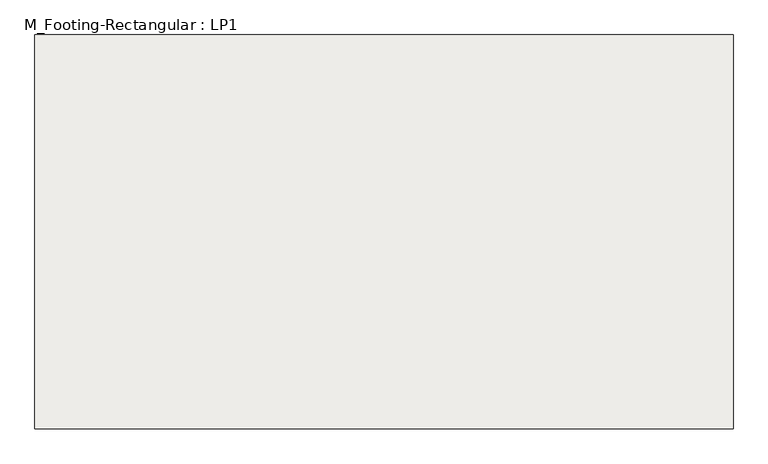
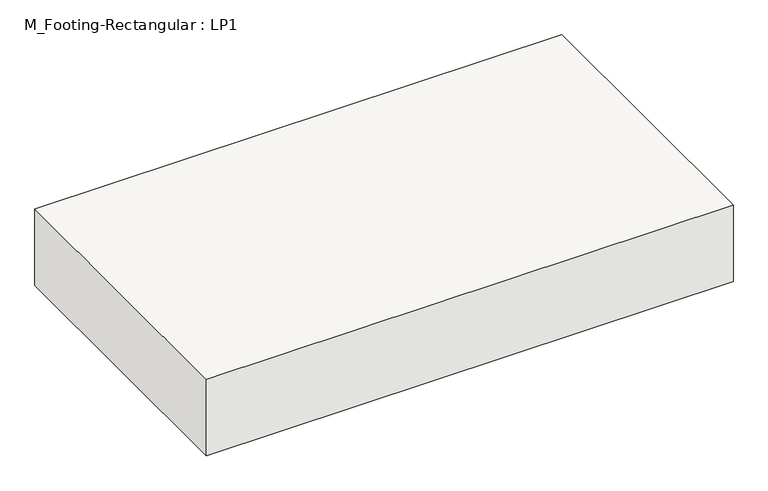
"""IFC4 building model written with IfcOpenShell, lengths in millimetres: slab geometry, M_Footing-Rectangular : LP1."""

from ifc_helpers import new_model, si_unit, frame, origin, place, context, project, spatial, polyline, outline, extrude, source, transform, mapped, element, save


def m_footing_rectangular_lp1_02c7f121(model_context):
    return source(origin(), model_context, "Body", "SweptSolid", [
        extrude(outline(polyline([(1485.9, 838.2), (1485.9, -838.2), (-1485.9, -838.2), (-1485.9, 838.2), (1485.9, 838.2)])), frame((0.0, 0.0, -457.2), z_axis=(0.0, 0.0, 1.0), x_axis=(1.0, 0.0, 0.0)), (0.0, 0.0, 1.0), 457.2),
    ])


if __name__ == "__main__":
    model = new_model("IFC4")
    model_context = context("Model", 3, world=origin())
    ifc_project = project(units=[si_unit("LENGTHUNIT", "METRE", prefix="MILLI")], contexts=[model_context])
    site = spatial("IfcSite", under=ifc_project)
    building = spatial("IfcBuilding", under=site)
    placement = place(None, origin())
    m_footing_rectangular_lp1_shape = m_footing_rectangular_lp1_02c7f121(model_context)
    element("IfcSlab", 1, ObjectType="M_Footing-Rectangular : LP1", at=placement, inside=building, context=model_context, shape_type="MappedRepresentation", body=[
        mapped(m_footing_rectangular_lp1_shape, transform((0.0, 0.0, 0.0), x_axis=(1.0, 0.0, 0.0), y_axis=(0.0, 1.0, 0.0), z_axis=(0.0, 0.0, 1.0))),
    ])
    save(model, "model.ifc")

# Revit data of these elements
# Type "M_Footing-Rectangular : LP1"
#   Width = 2971.8 mm
#   Length = 1676.4 mm
#   Foundation Thickness = 457.2 mm
#   Structural Material [instance default] = Concrete, Cast-in-Place gray
#   Assembly Code = ""
# Element 1 (IfcSlab, "M_Footing-Rectangular : LP1")
#   Materials on its faces: "Concrete, Cast-in-Place gray"
# Materials
#   "Concrete, Cast-in-Place gray": class "Concrete", colour RGB 192 192 192, transparency 0, Description = "Cast-in-place concrete", Cost = 0
